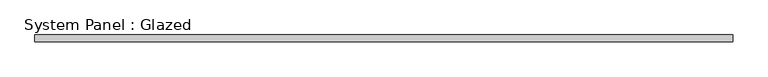
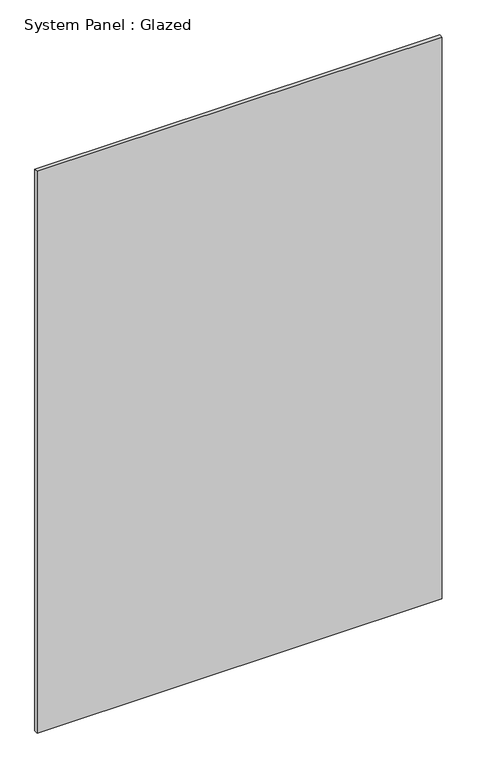
"""IFC4 building model written with IfcOpenShell, lengths in millimetres: plate geometry, System Panel : Glazed."""

from ifc_helpers import new_model, si_unit, origin, origin_with_axes, place, context, project, spatial, polyline, outline, extrude, source, transform, mapped, element, save


def system_panel_glazed_e9252991(model_context):
    return source(origin(), model_context, "Body", "SweptSolid", [
        extrude(outline(polyline([(1308.1, 19.05), (-1308.1, 19.05), (-1308.1, 44.45), (1308.1, 44.45), (1308.1, 19.05)])), origin_with_axes(), (0.0, 0.0, 1.0), 3835.4),
    ])


if __name__ == "__main__":
    model = new_model("IFC4")
    model_context = context("Model", 3, world=origin())
    ifc_project = project(units=[si_unit("LENGTHUNIT", "METRE", prefix="MILLI")], contexts=[model_context])
    site = spatial("IfcSite", under=ifc_project)
    building = spatial("IfcBuilding", under=site)
    placement = place(None, origin())
    system_panel_glazed_shape = system_panel_glazed_e9252991(model_context)
    element("IfcPlate", 1, ObjectType="System Panel : Glazed", at=placement, inside=building, context=model_context, shape_type="MappedRepresentation", body=[
        mapped(system_panel_glazed_shape, transform((0.0, 0.0, 0.0), x_axis=(1.0, 0.0, 0.0), y_axis=(0.0, 1.0, 0.0), z_axis=(0.0, 0.0, 1.0))),
    ])
    save(model, "model.ifc")

# Revit data of these elements
# Type "System Panel : Glazed"
#   Construction Type Id = "GSP4R"
#   Analytic Construction = "1/8 in Pilkington single glazing"
#   Visual Light Transmittance = 0.9
#   Solar Heat Gain Coefficient = 0.86
#   Heat Transfer Coefficient (U) = 1.18115 BTU/(h·ft²·°F)
# Element 1 (IfcPlate, "System Panel : Glazed")
#   Materials on its faces: "Glass"
# Materials
#   "Glass": class "Glass", colour RGB 0 128 192, transparency 0.75, Description = "Soda Lime Glass", Cost = 0
